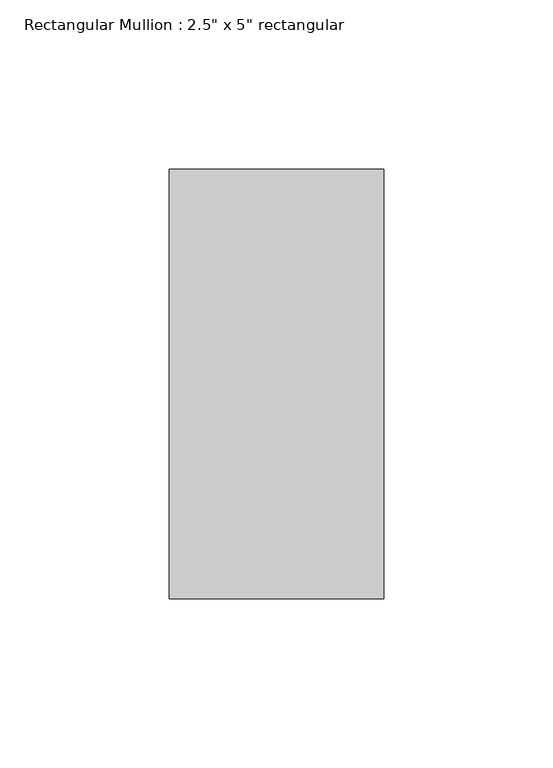
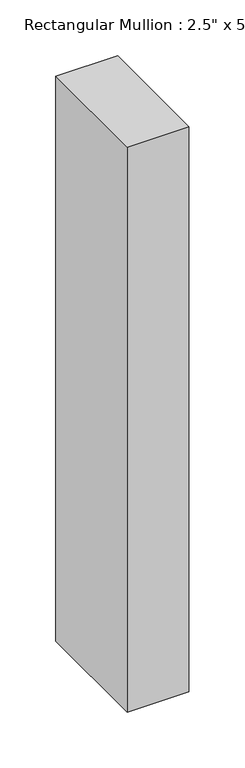
"""IFC4 building model written with IfcOpenShell, lengths in millimetres: member geometry."""

from ifc_helpers import new_model, si_unit, frame, origin, place, context, project, spatial, polyline, outline, extrude, source, transform, mapped, element, save


def member_3f0e0172(model_context):
    return source(origin(), model_context, "Body", "SweptSolid", [
        extrude(outline(polyline([(0.0, 63.5), (0.0, -63.5), (-63.5, -63.5), (-63.5, 63.5), (0.0, 63.5)])), frame((0.0, 0.0, -615.95), z_axis=(0.0, 0.0, 1.0), x_axis=(1.0, 0.0, 0.0)), (0.0, 0.0, 1.0), 615.95),
    ])


if __name__ == "__main__":
    model = new_model("IFC4")
    model_context = context("Model", 3, world=origin())
    ifc_project = project(units=[si_unit("LENGTHUNIT", "METRE", prefix="MILLI")], contexts=[model_context])
    site = spatial("IfcSite", under=ifc_project)
    building = spatial("IfcBuilding", under=site)
    placement = place(None, origin())
    member_shape = member_3f0e0172(model_context)
    element("IfcMember", 1, ObjectType="Rectangular Mullion : 2.5\" x 5\" rectangular", at=placement, inside=building, context=model_context, shape_type="MappedRepresentation", body=[
        mapped(member_shape, transform((0.0, 0.0, 0.0), x_axis=(1.0, 0.0, 0.0), y_axis=(0.0, 1.0, 0.0), z_axis=(0.0, 0.0, 1.0))),
    ])
    save(model, "model.ifc")

# Revit data of these elements
# Type "Rectangular Mullion : 2.5\" x 5\" rectangular"
#   built-in parameter 1007304 = 0.416667 (stored number, unit not read)
#   built-in parameter 1007301 = 0.104167 (stored number, unit not read)
#   built-in parameter 1007300 = 0.104167 (stored number, unit not read)
# Element 1 (IfcMember, "Rectangular Mullion : 2.5\" x 5\" rectangular")
#   Materials on its faces: "Aluminum"
# Materials
#   "Aluminum": class "Metal", colour RGB 247 247 247, transparency 0, Description = "Aluminum 6061", Cost = 0
